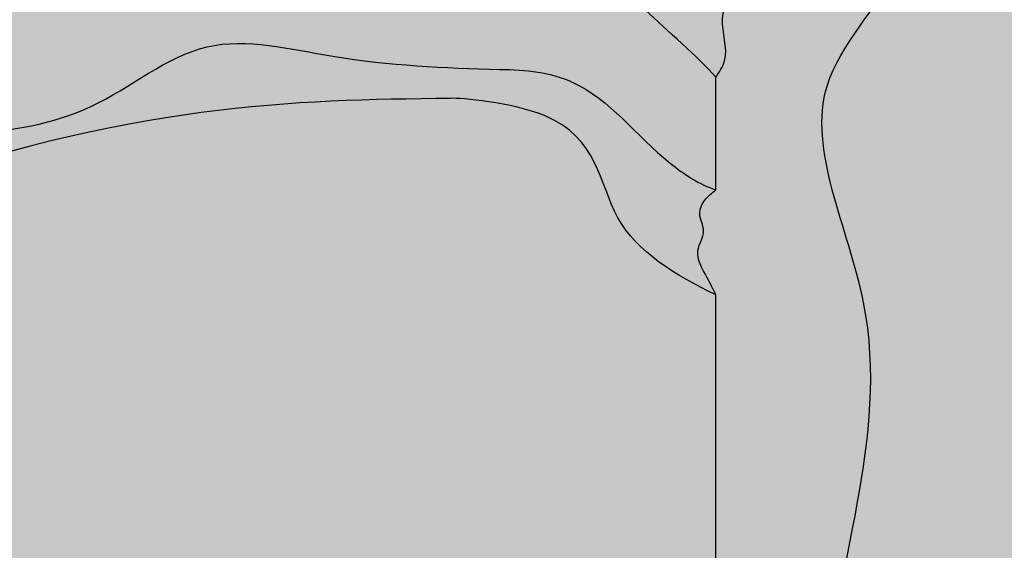
# Model space of a CAD drawing. Units: inches. Extents: x 1704 to 6393, y -157 to 1172.
# Tile 34 of 122: x 2548.79 to 2563.15, y 131.41 to 139.14. Entities that reach past the tile are written whole.
import ezdxf

# ---------------------------------------------------------------- set-up
doc = ezdxf.new("R2010")
doc.units = ezdxf.units.IN
doc.header["$MEASUREMENT"] = 0
for name, color, linetype, lineweight in [('A-ANNO-DIMS', 7, 'Continuous', 13), ('A-FURN', 8, 'Continuous', 18), ('estofado', 7, 'Continuous', 25)]:
    doc.layers.add(name, color=color, linetype=linetype, lineweight=lineweight)
doc.layers.add('A-FLOR-PATT', color=7, linetype='Continuous', lineweight=13, true_color=0xf2f2f2)
doc.styles.get("Standard").update_dxf_attribs({"font": 'arial.ttf'})
doc.dimstyles.get("Standard").update_dxf_attribs({"dimtxt": 6, "dimasz": 2, "dimexe": 0.18, "dimexo": 0.0625, "dimgap": 0.09, "dimtad": 0, "dimtih": 1, "dimtoh": 1, "dimdec": 1, "dimzin": 0, "dimdsep": 46, "dimlunit": 3, "dimtxsty": 'Standard', "dimblk": 'ARCHTICK', "dimcen": 0.09, "dimadec": 0, "dimazin": 0, "dimtfac": 1, "dimtdec": 1, "dimtofl": 0, "dimtmove": 0, "dimatfit": 3, "dimfxl": 1, "dimtolj": 1, "dimtzin": 0, "dimarcsym": 0})

# ---------------------------------------------------------------- blocks, each defined once
blk = doc.blocks.new('Cama Box Regencia LOLA')
at = {"layer": 'estofado', "ltscale": 0.2}
h = blk.add_hatch(color=256, dxfattribs=at)
h.dxf.hatch_style = 1
h.set_gradient(color1=(240, 232, 219), color2=(213, 190, 154), one_color=1, tint=0.7200000286102295)
edge = h.paths.add_edge_path()
edge.add_line((-0.8000000000000682, -0.1548023628405417), (-0.863597199697665, -0.2293271111754507))
edge.add_spline(control_points=[(-0.8635971996977787, -0.2293271111754507), (-0.8537222782123308, -0.258285373872468), (-0.8269013755602826, -0.3369378214810581), (-0.8674912876567759, -0.4595932758330151), (-0.8253488717912205, -0.6001498518888299), (-0.8771423076391329, -0.7139760714239288), (-0.8243323781925938, -0.8129899320257435), (-0.885044987287756, -0.8716602542656914), (-0.879518062107536, -0.9542863467743244), (-0.8339551707063037, -1.008464155856984), (-0.8245672924600739, -1.059984630119799), (-0.8208601923470268, -1.104655887174089), (-0.8073908324747662, -1.131238421004809), (-0.7999999999999546, -1.145824641594799)], knot_values=[0, 0, 0, 0, 0.0901802310564388, 0.2449351320798513, 0.3646438241986237, 0.5132330690395209, 0.5950634960661151, 0.646820388242338, 0.740988272125753, 0.8098674202588053, 0.8551784313864677, 0.8950360916221496, 0.9434986994854018, 0.9434986994854018, 0.9434986994854018, 0.9434986994854018], degree=3, periodic=0)
edge.add_line((-0.7999999999999546, -1.145824641594856), (-0.7999999999999546, -0.9571831923306604))
edge.add_spline(control_points=[(-0.8000000000001818, -0.9571831923294098), (-0.8003674620557603, -0.9560020588672273), (-0.8014778173377408, -0.9524330433489467), (-0.799534669348418, -0.9460450666617248), (-0.7963405736333016, -0.9382358308520792), (-0.7944188048602429, -0.9289040147384638), (-0.7953122817383474, -0.9190683391483389), (-0.7985341887020923, -0.9137677522519994), (-0.7999999999999546, -0.911356242470788)], knot_values=[0, 0, 0, 0, 0.0036609130031785, 0.0110621328900358, 0.0190316076023675, 0.0292873612819121, 0.0393286152452009, 0.0477100398955968, 0.0477100398955968, 0.0477100398955968, 0.0477100398955968], degree=3, periodic=0)
edge.add_line((-0.8000000000000682, -0.9113562424705037), (-0.7999999999999546, -0.8573491405791173))
edge.add_spline(control_points=[(-0.7999999999999546, -0.8573491405791173), (-0.8011509914009592, -0.8570771933481751), (-0.804102924754261, -0.8563797336621519), (-0.8039036519178353, -0.8498286502876908), (-0.8010279369466388, -0.8413595542568258), (-0.805623441450507, -0.8302818657685406), (-0.801318481758244, -0.8238273834048186), (-0.7999999999999546, -0.8218505664625013)], knot_values=[0, 0, 0, 0, 0.0032305881034183, 0.0082854491905874, 0.015951437769388, 0.0315866871777379, 0.0384893971878813, 0.0384893971878813, 0.0384893971878813, 0.0384893971878813], degree=3, periodic=0)
edge.add_line((-0.7999999999999546, -0.821850566462558), (-0.7999999999999546, -0.7800193173444541))
edge.add_spline(control_points=[(-0.7999999999999546, -0.7800193173443404), (-0.7985416092056994, -0.7788853679199974), (-0.7956241855360986, -0.7766169698310819), (-0.7929439183725436, -0.7707329795046576), (-0.7969680334608711, -0.7644035258254576), (-0.7912681985083055, -0.7566015403456845), (-0.7963938877088595, -0.7483952775559715), (-0.798936373489596, -0.7431699116222604), (-0.799999999999841, -0.7409839258539251)], knot_values=[0, 0, 0, 0, 0.0055481279082489, 0.0110986984731684, 0.0174746050947868, 0.0251556172852474, 0.035519246289823, 0.0429729849735991, 0.0429729849735991, 0.0429729849735991, 0.0429729849735991], degree=3, periodic=0)
edge.add_line((-0.7999999999999546, -0.740983925853584), (-0.8000000000000682, -0.1548023628405417))
h = blk.add_hatch(color=256, dxfattribs=at)
h.dxf.hatch_style = 1
h.set_gradient(color1=(240, 232, 219), color2=(213, 190, 154), one_color=1, tint=0.7200000286102295, name='CURVED')
edge = h.paths.add_edge_path()
edge.add_spline(control_points=[(0.343533776195045, -0.8455058148597345), (0.2879313990920309, -0.8167160606696484), (0.2054770794474052, -0.7744470032542381), (0.0954193394759386, -0.7742416952675626), (-0.0885363502328574, -0.7276964167006668), (0.2428192566063672, -0.7672518992321216), (0.345087521536243, -0.8076697826234067), (0.3825206986321063, -0.8228555492498799)], knot_values=[0.0056315103357428, 0.0056315103357428, 0.0056315103357428, 0.0056315103357428, 0.1860138916206105, 0.2660015162584448, 0.3570871810327863, 0.5963901805690979, 0.739731738908988, 0.739731738908988, 0.739731738908988, 0.739731738908988], degree=3, periodic=0)
edge.add_spline(control_points=[(0.3825206986325611, -0.8228555492497662), (0.3974221570828149, -0.8135511441712424), (0.4121061736600496, -0.8037181558521524), (0.4266849906532571, -0.7937075488799225)], knot_values=[1.358237767273279, 1.358237767273279, 1.358237767273279, 1.358237767273279, 1.409915662372559, 1.409915662372559, 1.409915662372559, 1.409915662372559], degree=3, periodic=0)
edge.add_spline(control_points=[(0.4266849905698109, -0.7937075489369932), (0.3998777739682282, -0.7821381809783361), (0.3476761897024971, -0.7634757898491671), (0.2670618099601825, -0.7565375622627358), (0.0835725072796549, -0.7192994417154637), (0.288524529784695, -0.7446405493717521), (0.4247448861246994, -0.7759943071475277), (0.4449816270193879, -0.7810438091316882)], knot_values=[0.1043639306803623, 0.1043639306803623, 0.1043639306803623, 0.1043639306803623, 0.1896363068641149, 0.2696239315019491, 0.3607095962762907, 0.6000125958126024, 0.6446217338078729, 0.6446217338078729, 0.6446217338078729, 0.6446217338078729], degree=3, periodic=0)
edge.add_spline(control_points=[(0.4449816270197289, -0.7810438091316882), (0.5029779388527232, -0.7406836481117695), (0.5966687145296419, -0.6736247633211292), (0.7071737530245628, -0.6656573253703187), (0.7517012483331201, -0.6672238302253392)], knot_values=[1.43159032281798, 1.43159032281798, 1.43159032281798, 1.43159032281798, 1.63814180148235, 1.770695287284994, 1.770695287284994, 1.770695287284994, 1.770695287284994], degree=3, periodic=0)
edge.add_arc((0.7481853615017826, -0.767162003811734), 0.0999999999999888, 58.7920033978138, 87.98512997550938, ccw=False)
edge.add_line((0.8000000000000682, -0.6816328085782289), (0.8000000000000682, -0.154802362840428))
edge.add_line((0.8000000000000682, -0.154802362840428), (-0.7999999999999546, -0.154802362840428))
edge.add_line((-0.7999999999999546, -0.154802362840428), (-0.8000000000000682, -0.7409839258539819))
edge.add_spline(control_points=[(-0.799999999999841, -0.7409839258539251), (-0.7846451382113174, -0.74846387981205), (-0.7568940913494089, -0.7651582159765554), (-0.7559936909002545, -0.8096905380045313), (-0.7049413305308008, -0.8142555457367848), (-0.7013836936888538, -0.8139988647640733)], knot_values=[0.0122267587020837, 0.0122267587020837, 0.0122267587020837, 0.0122267587020837, 0.0594720782072034, 0.1062176618094138, 0.134458043575382, 0.134458043575382, 0.134458043575382, 0.134458043575382], degree=3, periodic=0)
edge.add_spline(control_points=[(-0.7013836936890812, -0.8139988647637892), (-0.6428309483887916, -0.8132695376718857), (-0.532520673001045, -0.8118955240036598), (-0.2390712668254764, -0.6717984706609172), (-0.3892411364554391, -0.7557901092520752), (-0.4591093260188473, -0.8070101468627512), (-0.5571511178645779, -0.795652750469742), (-0.608497950975675, -0.8409486634728295), (-0.6632498050151981, -0.8266781836207997), (-0.6991149398675134, -0.8254126024436914), (-0.719552182989446, -0.8246914287938125)], knot_values=[0, 0, 0, 0, 0.2187005959148062, 0.4120203559900679, 0.4786136596093368, 0.6046444033330721, 0.6969970394608519, 0.7456449795902803, 0.7925683322559657, 0.8547274388453192, 0.8547274388453192, 0.8547274388453192, 0.8547274388453192], degree=3, periodic=0)
edge.add_spline(control_points=[(-0.7195521829781911, -0.824691428792164), (-0.7293124663336812, -0.8248308281530967), (-0.7545977292818407, -0.8216412233076653), (-0.7742556984202338, -0.794819860189591), (-0.7939222919129634, -0.7820064600295497), (-0.799999999999841, -0.7800193173443404)], knot_values=[0.1564883932805935, 0.1564883932805935, 0.1564883932805935, 0.1564883932805935, 0.184397548386913, 0.2313764834161266, 0.2505984550882281, 0.2505984550882281, 0.2505984550882281, 0.2505984550882281], degree=3, periodic=0)
edge.add_line((-0.8000000000000682, -0.7800193173444541), (-0.7999999999999546, -0.8218505664627286))
edge.add_spline(control_points=[(-0.7999999999999546, -0.8218505664625013), (-0.7938082505512511, -0.8290217081292894), (-0.7673857405620766, -0.8512914803976059), (-0.7619109683460011, -0.8661369353891359), (-0.6555700939965164, -0.8510070218793543), (-0.7139793977868294, -0.8637526923380391), (-0.7379026254519659, -0.8623504601624176), (-0.7688129786438367, -0.8813042143888196), (-0.7854260296310259, -0.8561610219318254), (-0.7961930533253962, -0.8566031243811949), (-0.7999999999999546, -0.8573491405791173)], knot_values=[0.0595743221876141, 0.0595743221876141, 0.0595743221876141, 0.0595743221876141, 0.08075289116965, 0.1037414994169835, 0.1697200936249022, 0.1760361327243865, 0.2071371586311508, 0.2404744334261798, 0.2623408547027293, 0.2736604507987723, 0.2736604507987723, 0.2736604507987723, 0.2736604507987723], degree=3, periodic=0)
edge.add_line((-0.7999999999999546, -0.8573491405791173), (-0.8000000000000682, -0.9113562424721521))
edge.add_spline(control_points=[(-0.8000000000000682, -0.9113562424720385), (-0.7937204054647964, -0.9077594990848183), (-0.7710343135782978, -0.8978798065321029), (-0.7213062468074442, -0.9144666877443228), (-0.6268586829058905, -0.862430497409548), (-0.6896594748232019, -0.9045634991654196), (-0.7483442493064559, -0.9189273406958591), (-0.7835301183422417, -0.922920432793262), (-0.7896301351460125, -0.9477657000142585), (-0.7975786973822779, -0.955260590410262), (-0.8000000000001818, -0.9571831923294098)], knot_values=[0.0138560263374175, 0.0138560263374175, 0.0138560263374175, 0.0138560263374175, 0.0348737775836104, 0.0888666909546002, 0.1078792274429341, 0.1267378491223226, 0.1587140219647659, 0.1937574699451985, 0.2174867851300671, 0.2267221218327879, 0.2267221218327879, 0.2267221218327879, 0.2267221218327879], degree=3, periodic=0)
edge.add_line((-0.7999999999999546, -0.957183192329296), (-0.7999999999999546, -1.145824641594742))
edge.add_spline(control_points=[(-0.8000000000002955, -1.145824641594913), (-0.7271039467997298, -1.094596787649038), (-0.4885706936571524, -0.9465888221489535), (-0.0701640902225336, -0.9707493165000187), (0.237911901821235, -0.902164522332157), (0.3435337762145991, -0.845505814843193)], knot_values=[0.1168958193629841, 0.1168958193629841, 0.1168958193629841, 0.1168958193629841, 0.3797203297758731, 0.9577018633805092, 1.31379338443587, 1.31379338443587, 1.31379338443587, 1.31379338443587], degree=3, periodic=0)
h.paths.add_polyline_path([(-0.6766340706021765, -0.6101327540145576, -0.3575266660906883), (-0.7312746368313583, -0.6354535276154252, -0.3575266660894137), (-0.7059538632299791, -0.5808129613865844, -0.1647847126465284), (-0.7059538632300928, -0.2676124402649407, -0.3575266660890756), (-0.7312746368312446, -0.2129718740360431, -0.3575266660908716), (-0.6766340706020629, -0.2382926476369676, -0.0925607043966334), (-0.1295169377724505, -0.2382926476369107, -0.3575266660898965), (-0.0748763715433825, -0.2129718740360431, -0.3575266660894428), (-0.1001971451446479, -0.2676124402649407, -0.1647847126465285), (-0.1001971451445343, -0.5808129613865844, -0.3575266660890756), (-0.0748763715433825, -0.6354535276154821, -0.3575266660898962), (-0.1295169377724505, -0.6101327540146145, -0.0925607043966531)], flags=16)
h.paths.add_polyline_path([(0.0748763715433825, -0.6354535276157094, -0.3575266660910266), (0.1001971451446479, -0.5808129613865844, -0.1647847126465284), (0.1001971451445343, -0.2676124402649407, -0.3575266660890757), (0.0748763715433825, -0.2129718740360431, -0.3575266660898962), (0.1295169377724505, -0.2382926476369107, -0.0925607043966334), (0.6766340706020629, -0.2382926476369676, -0.3575266660908718), (0.7312746368312446, -0.2129718740360431, -0.3575266660894425), (0.7059538632299791, -0.2676124402649407, -0.1647847126465283), (0.7059538632300928, -0.5808129613865844, -0.3575266660890756), (0.7312746368312446, -0.6354535276154821, -0.3575266660908716), (0.6766340706020629, -0.6101327540145576, -0.0925607043966335), (0.1295169377724505, -0.6101327540146145, -0.3575266660906303)], flags=16)
h = blk.add_hatch(color=256, dxfattribs=at)
h.dxf.hatch_style = 1
h.set_gradient(color1=(240, 232, 219), color2=(137, 106, 57), one_color=1, tint=0.3799999952316284, name='CURVED')
edge = h.paths.add_edge_path()
edge.add_spline(control_points=[(-0.719552182989446, -0.8246914287938125), (-0.6991149398675134, -0.8254126024436914), (-0.6632498050151981, -0.8266781836207997), (-0.608497950975675, -0.8409486634728295), (-0.5571511178645779, -0.795652750469742), (-0.4591093260188473, -0.8070101468627512), (-0.3892411364554391, -0.7557901092520752), (-0.2390712668254764, -0.6717984706609172), (-0.532520673001045, -0.8118955240036598), (-0.6428309483887916, -0.8132695376718857), (-0.7013836936890812, -0.8139988647637892)], knot_values=[0, 0, 0, 0, 0.0621591065893537, 0.1090824592550391, 0.1577303993844675, 0.2500830355122473, 0.3761137792359825, 0.4427070828552515, 0.6360268429305131, 0.8547274388453192, 0.8547274388453192, 0.8547274388453192, 0.8547274388453192], degree=3, periodic=0)
edge.add_spline(control_points=[(-0.7013836936888538, -0.8139988647640733), (-0.7049413305308008, -0.8142555457367848), (-0.7559936909002545, -0.8096905380045313), (-0.7568940913494089, -0.7651582159765554), (-0.7846451382113174, -0.74846387981205), (-0.799999999999841, -0.7409839258539251)], knot_values=[0.0122267587020837, 0.0122267587020837, 0.0122267587020837, 0.0122267587020837, 0.0404671404680519, 0.0872127240702623, 0.134458043575382, 0.134458043575382, 0.134458043575382, 0.134458043575382], degree=3, periodic=0)
edge.add_spline(control_points=[(-0.799999999999841, -0.7409839258539251), (-0.798936373489596, -0.7431699116222604), (-0.7963938877088595, -0.7483952775559715), (-0.7912681985083055, -0.7566015403456845), (-0.7969680334608711, -0.7644035258254576), (-0.7929439183725436, -0.7707329795046576), (-0.7956241855360986, -0.7766169698310819), (-0.7985416092056994, -0.7788853679199974), (-0.7999999999999546, -0.7800193173443404)], knot_values=[0, 0, 0, 0, 0.0074537386837761, 0.0178173676883516, 0.0254983798788123, 0.0318742865004307, 0.0374248570653501, 0.0429729849735991, 0.0429729849735991, 0.0429729849735991, 0.0429729849735991], degree=3, periodic=0)
edge.add_spline(control_points=[(-0.799999999999841, -0.7800193173443404), (-0.7939222919129634, -0.7820064600295497), (-0.7742556984202338, -0.794819860189591), (-0.7545977292818407, -0.8216412233076653), (-0.7293124663336812, -0.8248308281530967), (-0.7195521829781911, -0.824691428792164)], knot_values=[0.1564883932805935, 0.1564883932805935, 0.1564883932805935, 0.1564883932805935, 0.175710364952695, 0.2226892999819086, 0.2505984550882281, 0.2505984550882281, 0.2505984550882281, 0.2505984550882281], degree=3, periodic=0)
h = blk.add_hatch(color=256, dxfattribs=at)
h.dxf.hatch_style = 1
h.set_gradient(color1=(240, 232, 219), color2=(137, 106, 57), one_color=1, tint=0.3799999952316284, name='CURVED')
edge = h.paths.add_edge_path()
edge.add_spline(control_points=[(-0.7999999999999546, -0.8573491405791173), (-0.7961930533253962, -0.8566031243811949), (-0.7854260296310259, -0.8561610219318254), (-0.7688129786438367, -0.8813042143888196), (-0.7379026254519659, -0.8623504601624176), (-0.7139793977868294, -0.8637526923380391), (-0.6555700939965164, -0.8510070218793543), (-0.7619109683460011, -0.8661369353891359), (-0.7673857405620766, -0.8512914803976059), (-0.7938082505512511, -0.8290217081292894), (-0.7999999999999546, -0.8218505664625013)], knot_values=[0.0595743221876141, 0.0595743221876141, 0.0595743221876141, 0.0595743221876141, 0.0708939182836571, 0.0927603395602066, 0.1260976143552356, 0.1571986402619999, 0.1635146793614841, 0.2294932735694029, 0.2524818818167364, 0.2736604507987723, 0.2736604507987723, 0.2736604507987723, 0.2736604507987723], degree=3, periodic=0)
edge.add_spline(control_points=[(-0.7999999999999546, -0.8218505664625013), (-0.801318481758244, -0.8238273834048186), (-0.805623441450507, -0.8302818657685406), (-0.8010279369466388, -0.8413595542568258), (-0.8039036519178353, -0.8498286502876908), (-0.804102924754261, -0.8563797336621519), (-0.8011509914009592, -0.8570771933481751), (-0.7999999999999546, -0.8573491405791173)], knot_values=[0, 0, 0, 0, 0.0069027100101435, 0.0225379594184934, 0.030203947997294, 0.0352588090844631, 0.0384893971878813, 0.0384893971878813, 0.0384893971878813, 0.0384893971878813], degree=3, periodic=0)
for points in [[(0.8000000000000682, -0.6816328085741361), (0.8000000000000682, -0.154802362840428), (-0.7999999999999546, -0.154802362840428), (-0.7999999999999546, -0.7409839258540956)], [(-0.7999999999999546, -0.7800193173443404), (-0.7999999999999546, -0.8218505664625013)]]:
    blk.add_lwpolyline(points, dxfattribs=at)
for points, knots in [([(-0.8635971996977787, -0.2293271111754507), (-0.8537222782123597, -0.2582853738724713), (-0.8269013755602529, -0.3369378214810687), (-0.8674912876567628, -0.459593275832977), (-0.8253488717912105, -0.6001498518888299), (-0.8771423076387755, -0.7139760714238776), (-0.824332378192706, -0.8129899320257793), (-0.8850449872876955, -0.8716602542656513), (-0.8795180621076731, -0.9542863467744586), (-0.8339551707061605, -1.008464155856879), (-0.8245672924602526, -1.059984630119836), (-0.820860192346876, -1.104655887174075), (-0.8073908324747767, -1.131238421004865), (-0.7999999999999546, -1.145824641594799)], [0, 0, 0, 0, 0.0901802310564388, 0.2449351320798513, 0.3646438241986237, 0.5132330690395209, 0.5950634960661151, 0.646820388242338, 0.740988272125753, 0.8098674202588053, 0.8551784313864677, 0.8950360916221496, 0.9434986994854018, 0.9434986994854018, 0.9434986994854018, 0.9434986994854018]), ([(-0.7013836936890812, -0.8139988647637892), (-0.6428309483887775, -0.8132695376718778), (-0.5325206730010296, -0.8118955240036225), (-0.2390712668254173, -0.6717984706608711), (-0.3892411364555083, -0.755790109252117), (-0.4591093260187714, -0.8070101468627889), (-0.5571511178644899, -0.795652750469717), (-0.6084979509757439, -0.8409486634728317), (-0.6632498050152652, -0.8266781836208043), (-0.6991149398675783, -0.8254126024437319), (-0.719552182989446, -0.8246914287938125)], [0, 0, 0, 0, 0.2187005959148062, 0.4120203559900679, 0.4786136596093368, 0.6046444033330721, 0.6969970394608519, 0.7456449795902803, 0.7925683322559657, 0.8547274388453192, 0.8547274388453192, 0.8547274388453192, 0.8547274388453192]), ([(-0.799999999999841, -0.7409839258539251), (-0.7989363734895372, -0.7431699116222815), (-0.7963938877087565, -0.7483952775559015), (-0.7912681985084682, -0.7566015403457877), (-0.796968033460866, -0.7644035258254169), (-0.7929439183725189, -0.7707329795046354), (-0.7956241855361271, -0.7766169698311071), (-0.7985416092057079, -0.7788853679200344), (-0.7999999999999546, -0.7800193173443404)], [0, 0, 0, 0, 0.0074537386837761, 0.0178173676883516, 0.0254983798788123, 0.0318742865004307, 0.0374248570653501, 0.0429729849735991, 0.0429729849735991, 0.0429729849735991, 0.0429729849735991]), ([(-0.799999999999841, -0.7409839258539251), (-0.7846451382113174, -0.74846387981205), (-0.7568940913494089, -0.7651582159765554), (-0.7559936909002545, -0.8096905380045313), (-0.7049413305308008, -0.8142555457367848), (-0.7013836936888538, -0.8139988647640733)], [0.0122267587020837, 0.0122267587020837, 0.0122267587020837, 0.0122267587020837, 0.0594720782072034, 0.1062176618094138, 0.134458043575382, 0.134458043575382, 0.134458043575382, 0.134458043575382]), ([(-0.7195521829781911, -0.824691428792164), (-0.7293124663336812, -0.8248308281530967), (-0.7545977292818407, -0.8216412233076653), (-0.7742556984202338, -0.794819860189591), (-0.7939222919129634, -0.7820064600295497), (-0.799999999999841, -0.7800193173443404)], [0.1564883932805935, 0.1564883932805935, 0.1564883932805935, 0.1564883932805935, 0.184397548386913, 0.2313764834161266, 0.2505984550882281, 0.2505984550882281, 0.2505984550882281, 0.2505984550882281]), ([(-0.7999999999999546, -0.8218505664625013), (-0.8013184817582112, -0.8238273834047737), (-0.8056234414505565, -0.8302818657685486), (-0.8010279369466333, -0.8413595542568746), (-0.8039036519179351, -0.8498286502876482), (-0.80410292475424, -0.8563797336621606), (-0.8011509914010776, -0.857077193348196), (-0.7999999999999546, -0.8573491405791173)], [0, 0, 0, 0, 0.0069027100101435, 0.0225379594184934, 0.030203947997294, 0.0352588090844631, 0.0384893971878813, 0.0384893971878813, 0.0384893971878813, 0.0384893971878813]), ([(-0.7999999999999546, -0.8218505664625013), (-0.7938082505512511, -0.8290217081292894), (-0.7673857405620766, -0.8512914803976059), (-0.7619109683460011, -0.8661369353891359), (-0.6555700939965164, -0.8510070218793543), (-0.7139793977868294, -0.8637526923380391), (-0.7379026254519659, -0.8623504601624176), (-0.7688129786438367, -0.8813042143888196), (-0.7854260296310259, -0.8561610219318254), (-0.7961930533253962, -0.8566031243811949), (-0.7999999999999546, -0.8573491405791173)], [0.0595743221876141, 0.0595743221876141, 0.0595743221876141, 0.0595743221876141, 0.08075289116965, 0.1037414994169835, 0.1697200936249022, 0.1760361327243865, 0.2071371586311508, 0.2404744334261798, 0.2623408547027293, 0.2736604507987723, 0.2736604507987723, 0.2736604507987723, 0.2736604507987723])]:
    blk.add_open_spline(points, degree=3, knots=knots, dxfattribs=at)
blk = doc.blocks.new('_ArchTick')
at = {"color": 0, "linetype": 'ByBlock', "const_width": 0.15}
blk.add_lwpolyline([(-0.5, -0.5), (0.5, 0.5)], dxfattribs=at)
blk = doc.blocks.new('*D93')
at = {"layer": 'A-ANNO-DIMS', "color": 0, "lineweight": -2, "transparency": 16777216}
for p, q in [((2605.286074000001, 895.2129740000005), (1829.697551000002, 895.2129740000003)), ((1829.877551000002, 895.2129740000003), (1829.877551000002, 495.8664119263302)), ((1829.877551000002, 90.2129739999999), (1829.877551000002, 489.5595360736699)), ((2605.286074000001, 90.21297400000003), (1829.697551000002, 90.2129739999999))]:
    blk.add_line(p, q, dxfattribs=at)
at = {"layer": 'Defpoints', "color": 0, "lineweight": -3, "transparency": 16777216}
for p in [(2605.348574000001, 895.2129740000005), (1829.877551000002, 90.2129739999999), (2605.348574000001, 90.21297400000003)]:
    blk.add_point(p, dxfattribs=at)
at = {"layer": 'A-ANNO-DIMS', "color": 0, "lineweight": -2, "transparency": 16777216, "xscale": 2, "yscale": 2, "zscale": 2}
for p, rotation in [((1829.877551000002, 895.2129740000003), 90), ((1829.877551000002, 90.2129739999999), 270)]:
    blk.add_blockref('_ArchTick', p, dxfattribs=dict(at, rotation=rotation))
at = {"layer": 'A-ANNO-DIMS', "color": 0, "transparency": 16777216, "insert": (1829.877551000001, 492.7129739999994), "char_height": 6, "attachment_point": 5}
blk.add_mtext('\\A1;805', dxfattribs=at)

msp = doc.modelspace()

# ---------------------------------------------------------------- hatches: boundary and pattern name
at = {"layer": 'A-FLOR-PATT', "transparency": 33554528}
h = msp.add_hatch(color=256, dxfattribs=at)
h.dxf.hatch_style = 1
h.paths.add_polyline_path([(2325.348574056059, 863.2129735309796), (2325.348574056059, 887.2129735309796), (2263.348574056059, 887.2129735309796), (2167.348574056059, 887.2129735309794), (2081.348574056061, 887.2129735309792), (2081.348574056061, 719.2129735309785), (2277.348574056059, 719.2129735309787), (2277.348574056059, 711.2129735309788), (2277.348574056059, 372.212973530979), (2349.348574056059, 372.212973530979), (2381.348574056059, 372.2129735309789), (2381.348574056059, 364.2129735309789), (2353.348574056059, 364.2129735309789), (2353.348574056059, 270.2129735309788), (2381.348574056059, 270.2129735309788), (2381.348574056059, 266.2129735309788), (2357.348574056059, 266.2129735309788), (2357.348574056059, 98.21297353097884), (2381.348574056059, 98.21297353097897), (2385.181056550604, 98.21297353097884), (2386.482186711948, 98.21297353097884), (2424.21496140017, 98.21297353097884), (2425.516091561514, 98.21297353097884), (2429.348574056059, 98.21297353097897), (2597.348574056059, 98.21297353097884), (2597.348574056059, 146.2129735309788), (2597.348574056059, 218.2129735309788), (2597.348574056059, 266.2129735309788), (2423.348574056059, 266.2129735309788), (2423.348574056059, 270.2129735309788), (2473.348574056059, 270.2129735309788), (2473.348574056059, 294.2129735309789), (2477.348574056059, 294.2129735309789), (2477.348574056059, 270.2129735309788), (2547.348574056059, 270.2129735309788), (2547.348574056059, 364.2129735309788), (2477.348574056059, 364.2129735309788), (2477.348574056059, 318.2129735309788), (2473.348574056059, 318.2129735309787), (2473.348574056059, 364.2129735309789), (2423.348574056059, 364.2129735309788), (2423.348574056059, 372.2129735309788), (2469.348574056059, 372.2129735309788), (2469.348574056059, 459.2129735309789), (2469.348574056059, 538.2129735309788), (2350.348574056059, 538.2129735309788), (2350.348574056059, 565.7129735309788), (2358.348574056059, 565.7129735309788), (2358.348574056059, 545.2129735309788), (2420.348574056059, 545.2129735309788), (2420.348574056059, 610.2129735309788), (2358.348574056059, 610.2129735309788), (2358.348574056059, 589.7129735309788), (2350.348574056059, 589.7129735309788), (2350.348574056059, 615.2129735309788), (2425.348574056059, 615.2129735309788), (2425.348574056059, 607.2129735309788), (2425.348574056059, 546.2129735309788), (2469.348574056059, 546.2129735309788), (2514.34857405606, 546.212973530979), (2514.34857405606, 607.2129735309788), (2449.348574056059, 607.2129735309788), (2449.348574056059, 615.2129735309788), (2451.737974987759, 615.2129735309788), (2451.737974987759, 659.2129735309788), (2427.737974987759, 659.2129735309788), (2427.737974987759, 665.2129735309788), (2367.737974987758, 665.2129735309788), (2367.737974987758, 667.2129735309788), (2367.737974987758, 711.2129735309788), (2325.348574056059, 711.2129735309788), (2325.348574056059, 719.2129735309785), (2325.348574056059, 755.2129735309787), (2325.348574056059, 763.2129735309788)])
h.paths.add_polyline_path([(2233.85817000392, 822.532660166629, -0.1872470486944155), (2233.85817000392, 809.1396667958562), (2231.697030374885, 808.8044951349628, 0.0848927708004382), (2233.130501812631, 814.4858417746204), (2230.423974436808, 814.4858417746204, -0.1042581087707907), (2228.553363812687, 808.3129425443484), (2217.750790159711, 807.1555239386723, -0.2222222222222219), (2217.750790159711, 824.5168030238124), (2228.553363812687, 823.3593844181363, -0.1042581087707933), (2230.423974436808, 817.1864851878643), (2233.130501812631, 817.1864851878643, 0.08489277080044), (2231.697030374885, 822.8678318275219)], flags=16)
h.paths.add_polyline_path([(2213.621360876743, 833.1974425663823), (2213.621360876743, 798.4748843961024), (2156.047684459484, 798.4748843961034), (2156.047684459485, 833.1974425663813)], flags=16)
h.paths.add_polyline_path([(2203.931929661768, 848.0987249710489), (2205.089348267444, 837.2961513180724, -0.2222222222222264), (2187.728069182304, 837.2961513180724), (2188.88548778798, 848.0987249710485, -0.104258108770792), (2195.058387018252, 849.9693355951691), (2195.058387018252, 852.6758629709927, 0.084892770800438), (2189.377040378595, 851.2423915332469), (2189.712212039488, 853.4035311622828, -0.1872470486944166), (2203.105205410261, 853.4035311622828), (2203.440377071154, 851.2423915332469, 0.084892770800438), (2197.759030431496, 852.6758629709927), (2197.759030431496, 849.9693355951691, -0.1042581087707896)], flags=16)
h.paths.add_polyline_path([(2181.940976153924, 837.2961513180726, -0.2222222222222323), (2164.579697068783, 837.2961513180724), (2165.73711567446, 848.0987249710487, -0.1042581087707905), (2171.910014904732, 849.9693355951691), (2171.910014904732, 852.6758629709927, 0.0848927708004445), (2166.228668265074, 851.2423915332469), (2166.563839925967, 853.403531162283, -0.1872470486944096), (2179.95683329674, 853.4035311622828), (2180.292004957633, 851.2423915332465, 0.0848927708004458), (2174.610658317976, 852.6758629709927), (2174.610658317976, 849.9693355951691, -0.104258108770801), (2180.783557548248, 848.0987249710482)], flags=16)
h.paths.add_polyline_path([(2205.089348267444, 794.376175644412), (2203.931929661768, 783.5736019914364, -0.1042581087707934), (2197.759030431496, 781.7029913673155), (2197.759030431496, 778.9964639914921, 0.084892770800439), (2203.440377071154, 780.4299354292382), (2203.105205410261, 778.2687958002022, -0.1872470486944172), (2189.712212039488, 778.2687958002018), (2189.377040378595, 780.4299354292377, 0.0848927708004369), (2195.058387018252, 778.9964639914919), (2195.058387018252, 781.7029913673153, -0.1042581087707904), (2188.88548778798, 783.5736019914358), (2187.728069182304, 794.3761756444126, -0.2222222222222231)], flags=16)
h.paths.add_polyline_path([(2181.940976153924, 794.376175644412), (2180.783557548248, 783.5736019914364, -0.1042581087708008), (2174.610658317976, 781.7029913673153), (2174.610658317976, 778.9964639914921, 0.0848927708004458), (2180.292004957633, 780.4299354292382), (2179.95683329674, 778.268795800202, -0.1872470486944096), (2166.563839925967, 778.2687958002018), (2166.228668265074, 780.4299354292378, 0.0848927708004446), (2171.910014904732, 778.9964639914919), (2171.910014904732, 781.7029913673153, -0.1042581087707904), (2165.73711567446, 783.5736019914358), (2164.579697068783, 794.3761756444123, -0.2222222222222294)], flags=16)
h.paths.add_polyline_path([(2151.918255176517, 807.1555239386723), (2141.115681523541, 808.3129425443484, -0.1042581087707911), (2139.24507089942, 814.4858417746204), (2136.538543523597, 814.4858417746204, 0.08489277080044), (2137.972014961343, 808.8044951349626), (2135.810875332307, 809.1396667958562, -0.1872470486944109), (2135.810875332307, 822.5326601666285), (2137.972014961343, 822.8678318275221, 0.0848927708004416), (2136.538543523597, 817.1864851878643), (2139.24507089942, 817.1864851878643, -0.104258108770793), (2141.115681523541, 823.3593844181363), (2151.918255176517, 824.5168030238124, -0.2222222222222205)], flags=16)
h.paths.add_polyline_path([(2357.868011454448, 363.4102250290031), (2358.813881560335, 363.4102250290031, 0.7537604849588476)], flags=16)
h.paths.add_polyline_path([(2372.241054283868, 363.1167008961685), (2372.248110816919, 363.1167008961685), (2372.248110816919, 363.3425764997267), (2371.30224071103, 363.3425764997267), (2371.30224071103, 363.1392706554335, -1.360391292333951)], flags=16)
h.paths.add_polyline_path([(2371.309297244092, 272.7157694655011), (2371.30224071103, 272.7157694655011), (2371.30224071103, 272.4898938619428), (2372.248110816919, 272.4898938619428), (2372.248110816919, 272.6931997062759, -1.360391292393621)], flags=16)
h.paths.add_polyline_path([(2357.875067987504, 272.7157694655011), (2357.868011454452, 272.7157694655011), (2357.868011454452, 272.4898938619428), (2358.813881560341, 272.4898938619428), (2358.813881560341, 272.6931997062361, -1.360391292333948)], flags=16)
h.paths.add_polyline_path([(2353.768696905258, 363.0736921025416), (2376.347425366111, 363.0736921025416), (2376.347425366111, 272.7587782591281), (2353.768696905258, 272.7587782591281)], flags=16)
h.paths.add_polyline_path([(2354.772195947961, 362.0701930598379), (2375.343926323407, 362.0701930598379), (2375.343926323407, 273.7622773018316), (2354.772195947961, 273.7622773018318)], flags=0)
h.paths.add_polyline_path([(2357.868011454452, 363.3425764997267), (2358.813881560341, 363.3425764997266), (2358.813881560341, 363.1167008961684), (2357.868011454452, 363.1167008961684)], flags=16)
h.paths.add_polyline_path([(2359.287941640134, 359.1843485433627), (2359.287941640134, 360.0631949744305), (2370.828180631237, 360.0631949744362), (2370.828180631237, 359.1843485433769), (2374.332057422314, 359.1843485433812), (2374.332057422312, 358.4635369582513), (2372.835178716611, 358.4635369582524), (2372.835178716611, 357.5410357047662), (2374.332057422314, 357.5410357047678), (2374.332057422312, 356.8202241196381), (2372.835178716611, 356.820224119639), (2372.835178716611, 355.897722866153), (2374.332057422314, 355.8977228661546), (2374.332057422312, 355.1769112810248), (2372.835178716611, 355.1769112810259), (2372.835178716611, 354.2544100275397), (2374.332057422334, 354.2544100275415), (2374.332057422331, 353.5335984424117), (2372.835178716631, 353.5335984424126), (2372.835178716631, 352.6110971889265), (2374.332057422334, 352.6110971889282), (2374.332057422331, 351.8902856037984), (2372.835178716631, 351.8902856037993), (2372.835178716631, 350.9677843503132), (2374.332057422334, 350.967784350315), (2374.332057422331, 350.2469727651852), (2372.835178716631, 350.2469727651861), (2372.835178716631, 349.3244715117), (2374.332057422334, 349.3244715117017), (2374.332057422331, 348.603659926572), (2372.835178716631, 348.6036599265729), (2372.835178716631, 347.6811586730868), (2374.332057422334, 347.6811586730886), (2374.332057422331, 346.9603470879587), (2372.835178716631, 346.9603470879598), (2372.835178716631, 346.0378458344735), (2374.332057422334, 346.0378458344753), (2374.332057422331, 345.3170342493456), (2372.835178716631, 345.3170342493465), (2372.835178716631, 344.3945329958605), (2374.332057422334, 344.3945329958621), (2374.332057422331, 343.6737214107324), (2372.835178716631, 343.6737214107334), (2372.835178716631, 342.751220157247), (2374.332057422334, 342.7512201572489), (2374.332057422331, 342.0304085721191), (2372.835178716631, 342.03040857212), (2372.835178716631, 341.1079073186338), (2374.332057422334, 341.1079073186356), (2374.332057422331, 340.3870957335057), (2372.835178716631, 340.3870957335066), (2372.835178716631, 339.4645944800207), (2374.332057422334, 339.4645944800223), (2374.332057422331, 338.7437828948924), (2372.835178716648, 338.7437828948933), (2372.835178716648, 337.8212816414076), (2374.332057422334, 337.8212816414093), (2374.332057422331, 337.1004700562794), (2372.835178716648, 337.1004700562803), (2372.835178716648, 336.1779688027942), (2374.332057422334, 336.1779688027961), (2374.332057422331, 335.4571572176662), (2372.835178716648, 335.4571572176673), (2372.835178716648, 334.5346559641809), (2374.332057422334, 334.5346559641828), (2374.332057422331, 333.8138443790529), (2372.835178716648, 333.8138443790539), (2372.835178716648, 332.8913431255679), (2374.332057422334, 332.8913431255696), (2374.332057422331, 332.1705315404397), (2372.835178716648, 332.1705315404406), (2372.835178716648, 331.2480302869545), (2374.332057422334, 331.2480302869563), (2374.332057422331, 330.5272187018265), (2372.835178716648, 330.5272187018273), (2372.835178716648, 329.6047174483413), (2374.332057422334, 329.6047174483431), (2374.332057422331, 328.8839058632133), (2372.835178716648, 328.8839058632143), (2372.835178716648, 327.9614046097282), (2374.332057422334, 327.9614046097298), (2374.332057422331, 327.2405930246), (2372.835178716648, 327.2405930246009), (2372.835178716648, 326.3180917711149), (2374.332057422334, 326.3180917711167), (2374.332057422331, 325.5972801859869), (2372.835178716648, 325.5972801859877), (2372.835178716648, 324.6747789325016), (2374.332057422334, 324.6747789325034), (2374.332057422331, 323.9539673473736), (2372.835178716648, 323.9539673473746), (2372.835178716648, 323.0314660938884), (2374.332057422334, 323.0314660938901), (2374.332057422331, 322.3106545087603), (2372.835178716648, 322.3106545087613), (2372.835178716648, 321.3881532552753), (2374.332057422334, 321.388153255277), (2374.332057422331, 320.6673416701471), (2372.835178716648, 320.6673416701481), (2372.835178716648, 319.7448404166621), (2374.332057422334, 319.7448404166638), (2374.332057422331, 319.0240288315339), (2372.835178716648, 319.0240288315348), (2372.835178716648, 318.1015275780487), (2374.332057422334, 318.1015275780504), (2374.332057422331, 317.3807159929205), (2372.835178716648, 317.3807159929214), (2372.835178716648, 316.4582147394357), (2374.332057422334, 316.4582147394373), (2374.332057422331, 315.7374031543073), (2372.835178716648, 315.7374031543084), (2372.835178716648, 314.8149019008223), (2374.332057422334, 314.8149019008241), (2374.332057422331, 314.0940903156943), (2372.835178716648, 314.0940903156952), (2372.835178716648, 313.171589062209), (2374.332057422334, 313.1715890622108), (2374.332057422331, 312.450777477081), (2372.835178716648, 312.4507774770819), (2372.835178716648, 311.5282762235959), (2374.332057422334, 311.5282762235977), (2374.332057422331, 310.8074646384678), (2372.835178716648, 310.8074646384687), (2372.835178716648, 309.8849633849827), (2374.332057422334, 309.8849633849844), (2374.332057422331, 309.1641517998546), (2372.835178716648, 309.1641517998555), (2372.835178716648, 308.2416505463693), (2374.332057422334, 308.2416505463712), (2374.332057422331, 307.5208389612412), (2372.835178716648, 307.5208389612421), (2372.835178716648, 306.5983377077562), (2374.332057422334, 306.598337707758), (2374.332057422331, 305.8775261226281), (2372.835178716648, 305.8775261226289), (2372.835178716648, 304.955024869143), (2374.332057422334, 304.9550248691447), (2374.332057422331, 304.2342132840149), (2372.835178716648, 304.2342132840158), (2372.835178716648, 303.3117120305298), (2374.332057422334, 303.3117120305316), (2374.332057422331, 302.5909004454018), (2372.835178716648, 302.5909004454027), (2372.835178716648, 301.6683991919165), (2374.332057422334, 301.6683991919183), (2374.332057422331, 300.9475876067885), (2372.835178716648, 300.9475876067894), (2372.835178716648, 300.0250863533033), (2374.332057422334, 300.025086353305), (2374.332057422331, 299.3042747681752), (2372.835178716648, 299.3042747681761), (2372.835178716648, 298.3817735146902), (2374.332057422334, 298.3817735146919), (2374.332057422331, 297.6609619295621), (2372.835178716648, 297.6609619295629), (2372.835178716648, 296.7384606760769), (2374.332057422334, 296.7384606760786), (2374.332057422331, 296.0176490909488), (2372.835178716648, 296.0176490909498), (2372.835178716648, 295.0951478374636), (2374.332057422334, 295.0951478374653), (2374.332057422331, 294.3743362523355), (2372.835178716648, 294.3743362523364), (2372.835178716648, 293.4518349988504), (2374.332057422334, 293.4518349988522), (2374.332057422331, 292.7310234137224), (2372.835178716648, 292.7310234137233), (2372.835178716648, 291.8085221602371), (2374.332057422334, 291.8085221602389), (2374.332057422331, 291.0877105751091), (2372.835178716648, 291.08771057511), (2372.835178716648, 290.165209321624), (2374.332057422334, 290.1652093216256), (2374.332057422331, 289.4443977364957), (2372.835178716648, 289.4443977364966), (2372.835178716648, 288.5218964830108), (2374.332057422334, 288.5218964830125), (2374.332057422331, 287.8010848978827), (2372.835178716648, 287.8010848978836), (2372.835178716648, 286.8785836443975), (2374.332057422334, 286.8785836443993), (2374.332057422331, 286.1577720592695), (2372.835178716648, 286.1577720592703), (2372.835178716648, 285.2352708057842), (2374.332057422334, 285.2352708057861), (2374.332057422331, 284.5144592206562), (2372.835178716648, 284.514459220657), (2372.835178716648, 283.5919579671712), (2374.332057422334, 283.5919579671728), (2374.332057422331, 282.871146382043), (2372.835178716648, 282.8711463820439), (2372.835178716648, 281.9486451285579), (2374.332057422334, 281.9486451285596), (2374.332057422331, 281.2278335434298), (2372.835178716648, 281.2278335434307), (2372.835178716648, 280.3053322899446), (2374.332057422334, 280.3053322899464), (2374.332057422331, 279.5845207048164), (2372.835178716648, 279.5845207048174), (2372.835178716648, 278.6620194513314), (2374.332057422334, 278.6620194513331), (2374.332057422331, 277.9412078662033), (2372.835178716648, 277.9412078662043), (2372.835178716648, 277.0187066127184), (2374.332057422334, 277.0187066127201), (2374.332057422331, 276.29789502759), (2370.828180631244, 276.2978950275922), (2370.828180631244, 275.7692753872335), (2359.287941640128, 275.7692753872392), (2359.287941640128, 276.2978950275993), (2355.784064849037, 276.2978950276015), (2355.784064849037, 277.0187066126971), (2357.280943554723, 277.0187066126989), (2357.280943554723, 277.9412078662137), (2355.784064849037, 277.9412078662145), (2355.784064849037, 278.6620194513103), (2357.280943554723, 278.6620194513122), (2357.280943554723, 279.5845207048271), (2355.784064849037, 279.584520704828), (2355.784064849037, 280.3053322899236), (2357.280943554723, 280.3053322899253), (2357.280943554723, 281.2278335434403), (2355.784064849037, 281.2278335434412), (2355.784064849037, 281.9486451285369), (2357.280943554723, 281.9486451285387), (2357.280943554723, 282.8711463820535), (2355.784064849037, 282.8711463820543), (2355.784064849037, 283.5919579671501), (2357.280943554723, 283.591957967152), (2357.280943554723, 284.5144592206668), (2355.784064849037, 284.5144592206676), (2355.784064849037, 285.2352708057632), (2357.280943554723, 285.2352708057651), (2357.280943554723, 286.1577720592801), (2355.784064849037, 286.1577720592809), (2355.784064849037, 286.8785836443766), (2357.280943554723, 286.8785836443784), (2357.280943554723, 287.8010848978931), (2355.784064849037, 287.8010848978941), (2355.784064849037, 288.5218964829895), (2357.280943554723, 288.5218964829913), (2357.280943554723, 289.4443977365064), (2355.784064849037, 289.4443977365072), (2355.784064849037, 290.1652093216029), (2357.280943554723, 290.1652093216047), (2357.280943554723, 291.0877105751197), (2355.784064849037, 291.0877105751206), (2355.784064849037, 291.8085221602161), (2357.280943554723, 291.8085221602179), (2357.280943554723, 292.7310234137328), (2355.784064849037, 292.7310234137337), (2355.784064849037, 293.4518349988293), (2357.280943554723, 293.451834998831), (2357.280943554723, 294.3743362523461), (2355.784064849037, 294.3743362523469), (2355.784064849037, 295.0951478374426), (2357.280943554723, 295.0951478374445), (2357.280943554723, 296.0176490909594), (2355.784064849037, 296.0176490909601), (2355.784064849037, 296.7384606760557), (2357.280943554723, 296.7384606760575), (2357.280943554723, 297.6609619295724), (2355.784064849037, 297.6609619295734), (2355.784064849037, 298.3817735146691), (2357.280943554723, 298.3817735146709), (2357.280943554723, 299.3042747681858), (2355.784064849037, 299.3042747681866), (2355.784064849037, 300.0250863532823), (2357.280943554723, 300.0250863532841), (2357.280943554723, 300.9475876067989), (2355.784064849037, 300.9475876067997), (2355.784064849037, 301.6683991918954), (2357.280943554723, 301.6683991918973), (2357.280943554723, 302.5909004454123), (2355.784064849037, 302.5909004454133), (2355.784064849037, 303.3117120305088), (2357.280943554723, 303.3117120305105), (2357.280943554723, 304.2342132840254), (2355.784064849037, 304.2342132840262), (2355.784064849037, 304.9550248691219), (2357.280943554723, 304.9550248691238), (2357.280943554723, 305.8775261226386), (2355.784064849037, 305.8775261226394), (2355.784064849037, 306.5983377077352), (2357.280943554723, 306.5983377077369), (2357.280943554723, 307.5208389612518), (2355.784064849037, 307.5208389612528), (2355.784064849037, 308.2416505463484), (2357.280943554723, 308.2416505463501), (2357.280943554723, 309.1641517998652), (2355.784064849037, 309.1641517998661), (2355.784064849037, 309.8849633849617), (2357.280943554723, 309.8849633849634), (2357.280943554723, 310.8074646384782), (2355.784064849037, 310.8074646384791), (2355.784064849037, 311.5282762235748), (2357.280943554723, 311.5282762235767), (2357.280943554723, 312.4507774770916), (2355.784064849037, 312.4507774770925), (2355.784064849037, 313.171589062188), (2357.280943554723, 313.1715890621898), (2357.280943554723, 314.0940903157049), (2355.784064849037, 314.0940903157058), (2355.784064849037, 314.8149019008013), (2357.280943554723, 314.8149019008032), (2357.280943554723, 315.7374031543179), (2355.784064849037, 315.7374031543187), (2355.784064849037, 316.4582147394146), (2357.280943554723, 316.4582147394165), (2357.280943554723, 317.3807159929311), (2355.784064849037, 317.3807159929321), (2355.784064849037, 318.1015275780277), (2357.280943554723, 318.1015275780295), (2357.280943554723, 319.0240288315445), (2355.784064849037, 319.0240288315454), (2355.784064849037, 319.744840416641), (2357.280943554723, 319.7448404166428), (2357.280943554723, 320.6673416701576), (2355.784064849037, 320.6673416701585), (2355.784064849037, 321.3881532552541), (2357.280943554723, 321.388153255256), (2357.280943554723, 322.3106545087708), (2355.784064849037, 322.3106545087718), (2355.784064849037, 323.0314660938674), (2357.280943554723, 323.0314660938692), (2357.280943554723, 323.9539673473843), (2355.784064849037, 323.9539673473851), (2355.784064849037, 324.6747789324806), (2357.280943554723, 324.6747789324824), (2357.280943554723, 325.5972801859974), (2355.784064849037, 325.5972801859983), (2355.784064849037, 326.3180917710939), (2357.280943554723, 326.3180917710958), (2357.280943554723, 327.2405930246105), (2355.784064849037, 327.2405930246113), (2355.784064849037, 327.9614046097071), (2357.280943554723, 327.961404609709), (2357.280943554723, 328.8839058632238), (2355.784064849037, 328.8839058632245), (2355.784064849037, 329.6047174483202), (2357.280943554723, 329.604717448322), (2357.280943554723, 330.527218701837), (2355.784064849037, 330.5272187018379), (2355.784064849037, 331.2480302869335), (2357.280943554723, 331.2480302869353), (2357.280943554723, 332.1705315404502), (2355.784064849037, 332.170531540451), (2355.784064849037, 332.8913431255468), (2357.280943554723, 332.8913431255486), (2357.280943554723, 333.8138443790634), (2355.784064849037, 333.8138443790642), (2355.784064849037, 334.5346559641599), (2357.280943554723, 334.5346559641618), (2357.280943554723, 335.4571572176767), (2355.784064849037, 335.4571572176776), (2355.784064849037, 336.1779688027732), (2357.280943554723, 336.177968802775), (2357.280943554723, 337.1004700562898), (2355.784064849037, 337.1004700562908), (2355.784064849037, 337.8212816413864), (2357.280943554723, 337.8212816413883), (2357.280943554723, 338.7437828949031), (2355.784064849037, 338.743782894904), (2355.784064849037, 339.4645944799996), (2357.280943554706, 339.4645944800013), (2357.280943554706, 340.3870957335163), (2355.784064849037, 340.3870957335173), (2355.784064849037, 341.1079073186129), (2357.280943554706, 341.1079073186146), (2357.280943554706, 342.0304085721296), (2355.784064849037, 342.0304085721304), (2355.784064849037, 342.7512201572262), (2357.280943554706, 342.751220157228), (2357.280943554706, 343.6737214107429), (2355.784064849037, 343.6737214107437), (2355.784064849037, 344.3945329958394), (2357.280943554706, 344.3945329958412), (2357.280943554706, 345.317034249356), (2355.784064849037, 345.3170342493569), (2355.784064849037, 346.0378458344526), (2357.280943554706, 346.0378458344544), (2357.280943554706, 346.9603470879692), (2355.784064849037, 346.9603470879701), (2355.784064849037, 347.6811586730658), (2357.280943554706, 347.6811586730677), (2357.280943554706, 348.6036599265824), (2355.784064849037, 348.6036599265833), (2355.784064849037, 349.324471511679), (2357.280943554706, 349.3244715116809), (2357.280943554706, 350.2469727651956), (2355.784064849037, 350.2469727651966), (2355.784064849037, 350.9677843502922), (2357.280943554706, 350.9677843502939), (2357.280943554706, 351.8902856038089), (2355.784064849037, 351.8902856038098), (2355.784064849037, 352.6110971889055), (2357.280943554706, 352.6110971889072), (2357.280943554706, 353.5335984424222), (2355.784064849037, 353.533598442423), (2355.784064849037, 354.2544100275187), (2357.280943554686, 354.2544100275204), (2357.280943554686, 355.1769112810354), (2355.784064849017, 355.1769112810362), (2355.784064849017, 355.897722866132), (2357.280943554686, 355.8977228661338), (2357.280943554686, 356.8202241196486), (2355.784064849017, 356.8202241196495), (2355.784064849017, 357.5410357047453), (2357.280943554686, 357.5410357047471), (2357.280943554686, 358.4635369582618), (2355.784064849017, 358.4635369582626), (2355.784064849017, 359.1843485433584)], flags=0)

# ---------------------------------------------------------------- block references
at = {"layer": 'A-FURN', "xscale": 39.22313671019584, "yscale": 39.22313671019584, "zscale": 39.22313671019584, "rotation": 180}
msp.add_blockref('Cama Box Regencia LOLA', (2527.569415053021, 106.0625493409584), dxfattribs=at)

# ---------------------------------------------------------------- dimensions: what is measured, and where the dimension line sits
at = {"layer": 'A-ANNO-DIMS'}
dim = msp.add_linear_dim(base=(1829.877551000002, 90.2129739999999), p1=(2605.348574000001, 895.212974), p2=(2605.348574000001, 90.21297399999999), angle=90, dimstyle='Standard', override={"dimdec": 0, "dimlfac": 1, "dimrnd": 0, "dimzin": 0, "dimdsep": 46, "dimlunit": 2}, dxfattribs=at)
dim.commit()
dim.dimension.update_dxf_attribs({"geometry": '*D93', "text_midpoint": (1829.877551000001, 492.7129739999994)})

doc.saveas('drawing.dxf')
